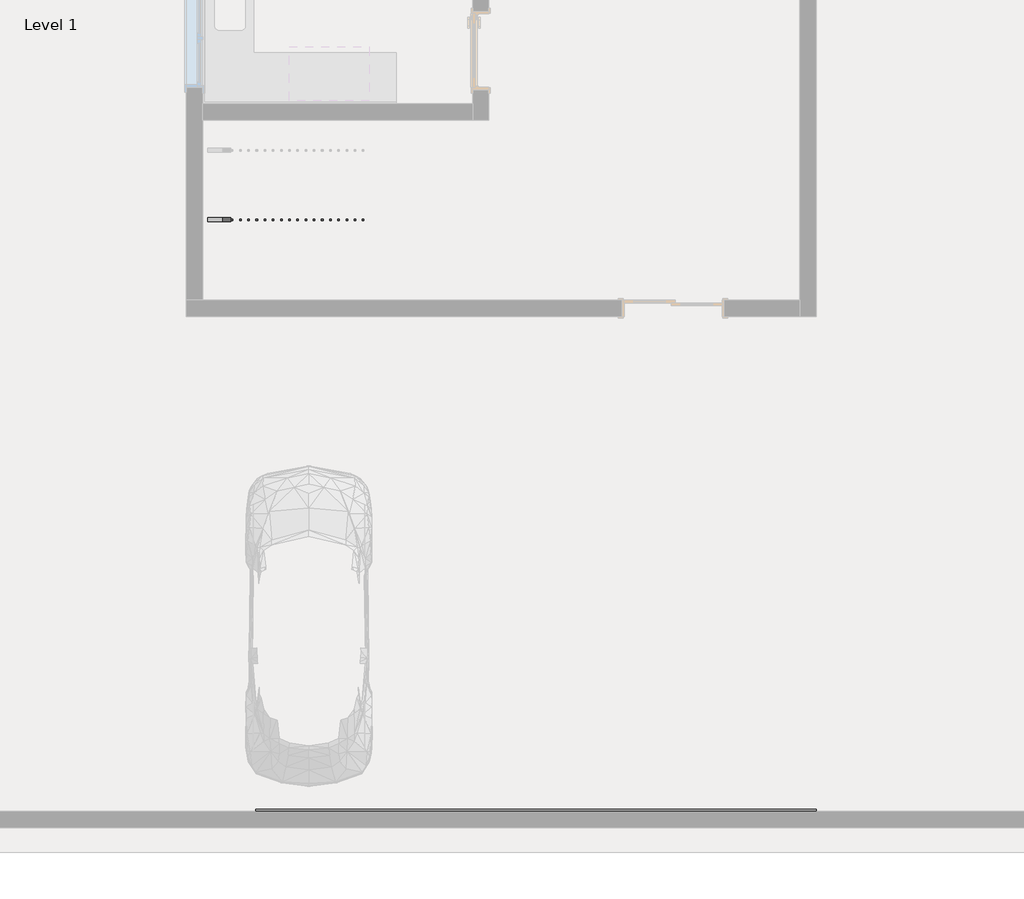
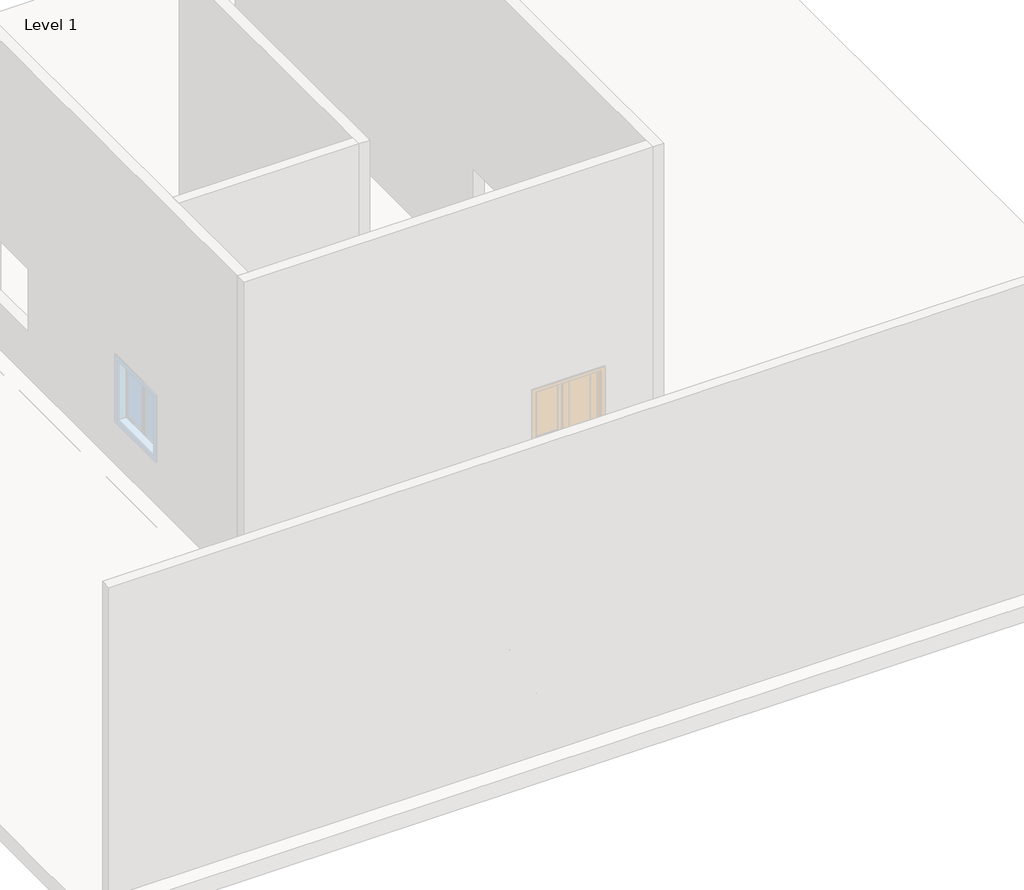
# One storey, part 2 of 3: 2 railings.
"""IFC4 building model written with IfcOpenShell, lengths in millimetres."""

from ifc_helpers import new_model, si_unit, frame, origin, origin_with_axes, place, context, project, spatial, polyline, outline, extrude, faceted_brep, element, save

model = new_model("IFC4")

# Units and contexts
model_context = context("Model", 3, world=origin())
ifc_project = project(units=[si_unit("LENGTHUNIT", "METRE", prefix="MILLI")], contexts=[model_context])

# Site, building, storey
site = spatial("IfcSite", under=ifc_project)
building = spatial("IfcBuilding", under=site)
storey = spatial("IfcBuildingStorey", under=building, Name="Level 1", Elevation=0.0)

# Railings
placement = place(None, origin())
element("IfcRailing", 1, ObjectType="Handrail - Rectangular", at=placement, inside=storey, context=model_context, shape_type="SolidModel", body=[
    faceted_brep([(-10833.7253666, -4140.9709044, 1090.3093851), (-10833.7253666, -4140.9709044, 1031.5187374), (-10833.7253666, -4191.7709044, 1031.5187374), (-10833.7253666, -4191.7709044, 1090.3093851), (-7938.1253666, -4140.9709044, 2777.0666667), (-7924.4080881, -4140.9709044, 2726.2666667), (-7924.4080881, -4191.7709044, 2726.2666667), (-7938.1253666, -4191.7709044, 2777.0666667), (-7499.9753666, -4140.9709044, 2777.0666667), (-7499.9753666, -4191.7709044, 2777.0666667), (-7449.1753666, -4191.7709044, 2726.2666667), (-7449.1753666, -4140.9709044, 2726.2666667)], [[[0, 1, 2, 3]], [[1, 0, 4, 5]], [[2, 1, 5, 6]], [[3, 2, 6, 7]], [[0, 3, 7, 4]], [[8, 9, 10, 11]], [[5, 4, 8, 11]], [[6, 5, 11, 10]], [[7, 6, 10, 9]], [[4, 7, 9, 8]]]),
    faceted_brep([(-7499.9753666, -4140.9709044, 2777.0666667), (-7499.9753666, -4090.1709044, 2777.0666667), (-7449.1753666, -4090.1709044, 2726.2666667), (-7449.1753666, -4140.9709044, 2726.2666667), (-7499.9753666, -4140.9709044, 3023.369697), (-7499.9753666, -4090.1709044, 2972.569697), (-7449.1753666, -4090.1709044, 2972.569697), (-7449.1753666, -4140.9709044, 3023.369697), (-7499.9753666, -4064.7709044, 3023.369697), (-7499.9753666, -4064.7709044, 2972.569697), (-7449.1753666, -4013.9709044, 2972.569697), (-7449.1753666, -4013.9709044, 3023.369697), (-7576.1753666, -4064.7709044, 3023.369697), (-7590.367776, -4064.7709044, 2972.569697), (-7590.367776, -4013.9709044, 2972.569697), (-7576.1753666, -4013.9709044, 3023.369697), (-9125.5753666, -4064.7709044, 3962.4), (-9125.5753666, -4013.9709044, 3962.4), (-9125.5753666, -4013.9709044, 3902.9985397), (-9125.5753666, -4064.7709044, 3902.9985397)], [[[0, 1, 2, 3]], [[1, 0, 4, 5]], [[2, 1, 5, 6]], [[3, 2, 6, 7]], [[0, 3, 7, 4]], [[5, 4, 8, 9]], [[6, 5, 9, 10]], [[7, 6, 10, 11]], [[4, 7, 11, 8]], [[9, 8, 12, 13]], [[10, 9, 13, 14]], [[11, 10, 14, 15]], [[8, 11, 15, 12]], [[16, 17, 18, 19]], [[13, 12, 16, 19]], [[14, 13, 19, 18]], [[15, 14, 18, 17]], [[12, 15, 17, 16]]]),
    extrude(outline(polyline([(3881.8318731, -9090.6503666), (3893.3773276, -9109.7003666), (2878.6666667, -9109.7003666), (2878.6666667, -9090.6503666), (3881.8318731, -9090.6503666)])), frame((0.0, -4048.8959044, 0.0), z_axis=(0.0, 1.0, 0.0), x_axis=(0.0, 0.0, 1.0)), (0.0, 0.0, 1.0), 19.05),
    extrude(outline(polyline([(3820.2561155, -8989.0503666), (3831.80157, -9008.1003666), (2878.6666667, -9008.1003666), (2878.6666667, -8989.0503666), (3820.2561155, -8989.0503666)])), frame((0.0, -4048.8959044, 0.0), z_axis=(0.0, 1.0, 0.0), x_axis=(0.0, 0.0, 1.0)), (0.0, 0.0, 1.0), 19.05),
    extrude(outline(polyline([(3758.6803579, -8887.4503666), (3770.2258125, -8906.5003666), (2878.6666667, -8906.5003666), (2878.6666667, -8887.4503666), (3758.6803579, -8887.4503666)])), frame((0.0, -4048.8959044, 0.0), z_axis=(0.0, 1.0, 0.0), x_axis=(0.0, 0.0, 1.0)), (0.0, 0.0, 1.0), 19.05),
    extrude(outline(polyline([(3697.1046004, -8785.8503666), (3708.6500549, -8804.9003666), (2709.3333333, -8804.9003666), (2709.3333333, -8785.8503666), (3697.1046004, -8785.8503666)])), frame((0.0, -4048.8959044, 0.0), z_axis=(0.0, 1.0, 0.0), x_axis=(0.0, 0.0, 1.0)), (0.0, 0.0, 1.0), 19.05),
    extrude(outline(polyline([(3635.5288428, -8684.2503666), (3647.0742973, -8703.3003666), (2709.3333333, -8703.3003666), (2709.3333333, -8684.2503666), (3635.5288428, -8684.2503666)])), frame((0.0, -4048.8959044, 0.0), z_axis=(0.0, 1.0, 0.0), x_axis=(0.0, 0.0, 1.0)), (0.0, 0.0, 1.0), 19.05),
    extrude(outline(polyline([(3573.9530852, -8582.6503666), (3585.4985397, -8601.7003666), (2709.3333333, -8601.7003666), (2709.3333333, -8582.6503666), (3573.9530852, -8582.6503666)])), frame((0.0, -4048.8959044, 0.0), z_axis=(0.0, 1.0, 0.0), x_axis=(0.0, 0.0, 1.0)), (0.0, 0.0, 1.0), 19.05),
    extrude(outline(polyline([(3512.3773276, -8481.0503666), (3523.9227822, -8500.1003666), (2540.0, -8500.1003666), (2540.0, -8481.0503666), (3512.3773276, -8481.0503666)])), frame((0.0, -4048.8959044, 0.0), z_axis=(0.0, 1.0, 0.0), x_axis=(0.0, 0.0, 1.0)), (0.0, 0.0, 1.0), 19.05),
    extrude(outline(polyline([(3450.80157, -8379.4503666), (3462.3470246, -8398.5003666), (2540.0, -8398.5003666), (2540.0, -8379.4503666), (3450.80157, -8379.4503666)])), frame((0.0, -4048.8959044, 0.0), z_axis=(0.0, 1.0, 0.0), x_axis=(0.0, 0.0, 1.0)), (0.0, 0.0, 1.0), 19.05),
    extrude(outline(polyline([(3389.2258125, -8277.8503666), (3400.771267, -8296.9003666), (2540.0, -8296.9003666), (2540.0, -8277.8503666), (3389.2258125, -8277.8503666)])), frame((0.0, -4048.8959044, 0.0), z_axis=(0.0, 1.0, 0.0), x_axis=(0.0, 0.0, 1.0)), (0.0, 0.0, 1.0), 19.05),
    extrude(outline(polyline([(3327.6500549, -8176.2503666), (3339.1955094, -8195.3003666), (2370.6666667, -8195.3003666), (2370.6666667, -8176.2503666), (3327.6500549, -8176.2503666)])), frame((0.0, -4048.8959044, 0.0), z_axis=(0.0, 1.0, 0.0), x_axis=(0.0, 0.0, 1.0)), (0.0, 0.0, 1.0), 19.05),
    extrude(outline(polyline([(3266.0742973, -8074.6503666), (3277.6197519, -8093.7003666), (2370.6666667, -8093.7003666), (2370.6666667, -8074.6503666), (3266.0742973, -8074.6503666)])), frame((0.0, -4048.8959044, 0.0), z_axis=(0.0, 1.0, 0.0), x_axis=(0.0, 0.0, 1.0)), (0.0, 0.0, 1.0), 19.05),
    extrude(outline(polyline([(3204.4985397, -7973.0503666), (3216.0439943, -7992.1003666), (2201.3333333, -7992.1003666), (2201.3333333, -7973.0503666), (3204.4985397, -7973.0503666)])), frame((0.0, -4048.8959044, 0.0), z_axis=(0.0, 1.0, 0.0), x_axis=(0.0, 0.0, 1.0)), (0.0, 0.0, 1.0), 19.05),
    extrude(outline(polyline([(3142.9227822, -7871.4503666), (3154.4682367, -7890.5003666), (2201.3333333, -7890.5003666), (2201.3333333, -7871.4503666), (3142.9227822, -7871.4503666)])), frame((0.0, -4048.8959044, 0.0), z_axis=(0.0, 1.0, 0.0), x_axis=(0.0, 0.0, 1.0)), (0.0, 0.0, 1.0), 19.05),
    extrude(outline(polyline([(3081.3470246, -7769.8503666), (3092.8924791, -7788.9003666), (2201.3333333, -7788.9003666), (2201.3333333, -7769.8503666), (3081.3470246, -7769.8503666)])), frame((0.0, -4048.8959044, 0.0), z_axis=(0.0, 1.0, 0.0), x_axis=(0.0, 0.0, 1.0)), (0.0, 0.0, 1.0), 19.05),
    extrude(outline(polyline([(3019.771267, -7668.2503666), (3031.3167216, -7687.3003666), (2032.0, -7687.3003666), (2032.0, -7668.2503666), (3019.771267, -7668.2503666)])), frame((0.0, -4048.8959044, 0.0), z_axis=(0.0, 1.0, 0.0), x_axis=(0.0, 0.0, 1.0)), (0.0, 0.0, 1.0), 19.05),
    extrude(outline(polyline([(-7566.6503666, -4029.8459044), (-7566.6503666, -4048.8959044), (-7585.7003666, -4048.8959044), (-7585.7003666, -4029.8459044), (-7566.6503666, -4029.8459044)])), frame((0.0, 0.0, 2032.0), z_axis=(0.0, 0.0, 1.0), x_axis=(1.0, 0.0, 0.0)), (0.0, 0.0, 1.0), 940.569697),
    extrude(outline(polyline([(-7465.0503666, -4074.2959044), (-7484.1003666, -4074.2959044), (-7484.1003666, -4055.2459044), (-7465.0503666, -4055.2459044), (-7465.0503666, -4074.2959044)])), frame((0.0, 0.0, 1862.6666667), z_axis=(0.0, 0.0, 1.0), x_axis=(1.0, 0.0, 0.0)), (0.0, 0.0, 1.0), 1109.9030303),
    extrude(outline(polyline([(-7541.2503666, -4175.8959044), (-7541.2503666, -4156.8459044), (-7522.2003666, -4156.8459044), (-7522.2003666, -4175.8959044), (-7541.2503666, -4175.8959044)])), frame((0.0, 0.0, 1862.6666667), z_axis=(0.0, 0.0, 1.0), x_axis=(1.0, 0.0, 0.0)), (0.0, 0.0, 1.0), 863.6),
    extrude(outline(polyline([(-7642.8503666, -4175.8959044), (-7642.8503666, -4156.8459044), (-7623.8003666, -4156.8459044), (-7623.8003666, -4175.8959044), (-7642.8503666, -4175.8959044)])), frame((0.0, 0.0, 1862.6666667), z_axis=(0.0, 0.0, 1.0), x_axis=(1.0, 0.0, 0.0)), (0.0, 0.0, 1.0), 863.6),
    extrude(outline(polyline([(-7744.4503666, -4175.8959044), (-7744.4503666, -4156.8459044), (-7725.4003666, -4156.8459044), (-7725.4003666, -4175.8959044), (-7744.4503666, -4175.8959044)])), frame((0.0, 0.0, 1862.6666667), z_axis=(0.0, 0.0, 1.0), x_axis=(1.0, 0.0, 0.0)), (0.0, 0.0, 1.0), 863.6),
    extrude(outline(polyline([(-7846.0503666, -4175.8959044), (-7846.0503666, -4156.8459044), (-7827.0003666, -4156.8459044), (-7827.0003666, -4175.8959044), (-7846.0503666, -4175.8959044)])), frame((0.0, 0.0, 1862.6666667), z_axis=(0.0, 0.0, 1.0), x_axis=(1.0, 0.0, 0.0)), (0.0, 0.0, 1.0), 863.6),
    extrude(outline(polyline([(2694.2323297, -7979.4003666), (2683.1352423, -7998.4503666), (1693.3333333, -7998.4503666), (1693.3333333, -7979.4003666), (2694.2323297, -7979.4003666)])), frame((0.0, -4175.8959044, 0.0), z_axis=(0.0, 1.0, 0.0), x_axis=(0.0, 0.0, 1.0)), (0.0, 0.0, 1.0), 19.05),
    extrude(outline(polyline([(2635.0478636, -8081.0003666), (2623.9507763, -8100.0503666), (1693.3333333, -8100.0503666), (1693.3333333, -8081.0003666), (2635.0478636, -8081.0003666)])), frame((0.0, -4175.8959044, 0.0), z_axis=(0.0, 1.0, 0.0), x_axis=(0.0, 0.0, 1.0)), (0.0, 0.0, 1.0), 19.05),
    extrude(outline(polyline([(2575.8633976, -8182.6003666), (2564.7663102, -8201.6503666), (1693.3333333, -8201.6503666), (1693.3333333, -8182.6003666), (2575.8633976, -8182.6003666)])), frame((0.0, -4175.8959044, 0.0), z_axis=(0.0, 1.0, 0.0), x_axis=(0.0, 0.0, 1.0)), (0.0, 0.0, 1.0), 19.05),
    extrude(outline(polyline([(2516.6789316, -8284.2003666), (2505.5818442, -8303.2503666), (1655.5210356, -8303.2503666), (1655.5210356, -8284.2003666), (2516.6789316, -8284.2003666)])), frame((0.0, -4175.8959044, 0.0), z_axis=(0.0, 1.0, 0.0), x_axis=(0.0, 0.0, 1.0)), (0.0, 0.0, 1.0), 19.05),
    extrude(outline(polyline([(2457.4944656, -8385.8003666), (2446.3973782, -8404.8503666), (1524.0, -8404.8503666), (1524.0, -8385.8003666), (2457.4944656, -8385.8003666)])), frame((0.0, -4175.8959044, 0.0), z_axis=(0.0, 1.0, 0.0), x_axis=(0.0, 0.0, 1.0)), (0.0, 0.0, 1.0), 19.05),
    extrude(outline(polyline([(2398.3099996, -8487.4003666), (2387.2129122, -8506.4503666), (1524.0, -8506.4503666), (1524.0, -8487.4003666), (2398.3099996, -8487.4003666)])), frame((0.0, -4175.8959044, 0.0), z_axis=(0.0, 1.0, 0.0), x_axis=(0.0, 0.0, 1.0)), (0.0, 0.0, 1.0), 19.05),
    extrude(outline(polyline([(2339.1255336, -8589.0003666), (2328.0284462, -8608.0503666), (1354.6666667, -8608.0503666), (1354.6666667, -8589.0003666), (2339.1255336, -8589.0003666)])), frame((0.0, -4175.8959044, 0.0), z_axis=(0.0, 1.0, 0.0), x_axis=(0.0, 0.0, 1.0)), (0.0, 0.0, 1.0), 19.05),
    extrude(outline(polyline([(2279.9410675, -8690.6003666), (2268.8439802, -8709.6503666), (1354.6666667, -8709.6503666), (1354.6666667, -8690.6003666), (2279.9410675, -8690.6003666)])), frame((0.0, -4175.8959044, 0.0), z_axis=(0.0, 1.0, 0.0), x_axis=(0.0, 0.0, 1.0)), (0.0, 0.0, 1.0), 19.05),
    extrude(outline(polyline([(2220.7566015, -8792.2003666), (2209.6595141, -8811.2503666), (1354.6666667, -8811.2503666), (1354.6666667, -8792.2003666), (2220.7566015, -8792.2003666)])), frame((0.0, -4175.8959044, 0.0), z_axis=(0.0, 1.0, 0.0), x_axis=(0.0, 0.0, 1.0)), (0.0, 0.0, 1.0), 19.05),
    extrude(outline(polyline([(2161.5721355, -8893.8003666), (2150.4750481, -8912.8503666), (1185.3333333, -8912.8503666), (1185.3333333, -8893.8003666), (2161.5721355, -8893.8003666)])), frame((0.0, -4175.8959044, 0.0), z_axis=(0.0, 1.0, 0.0), x_axis=(0.0, 0.0, 1.0)), (0.0, 0.0, 1.0), 19.05),
    extrude(outline(polyline([(2102.3876695, -8995.4003666), (2091.2905821, -9014.4503666), (1185.3333333, -9014.4503666), (1185.3333333, -8995.4003666), (2102.3876695, -8995.4003666)])), frame((0.0, -4175.8959044, 0.0), z_axis=(0.0, 1.0, 0.0), x_axis=(0.0, 0.0, 1.0)), (0.0, 0.0, 1.0), 19.05),
    extrude(outline(polyline([(2043.2032035, -9097.0003666), (2032.1061161, -9116.0503666), (1182.0453074, -9116.0503666), (1182.0453074, -9097.0003666), (2043.2032035, -9097.0003666)])), frame((0.0, -4175.8959044, 0.0), z_axis=(0.0, 1.0, 0.0), x_axis=(0.0, 0.0, 1.0)), (0.0, 0.0, 1.0), 19.05),
    extrude(outline(polyline([(1984.0187374, -9198.6003666), (1972.9216501, -9217.6503666), (1016.0, -9217.6503666), (1016.0, -9198.6003666), (1984.0187374, -9198.6003666)])), frame((0.0, -4175.8959044, 0.0), z_axis=(0.0, 1.0, 0.0), x_axis=(0.0, 0.0, 1.0)), (0.0, 0.0, 1.0), 19.05),
    extrude(outline(polyline([(1924.8342714, -9300.2003666), (1913.737184, -9319.2503666), (1016.0, -9319.2503666), (1016.0, -9300.2003666), (1924.8342714, -9300.2003666)])), frame((0.0, -4175.8959044, 0.0), z_axis=(0.0, 1.0, 0.0), x_axis=(0.0, 0.0, 1.0)), (0.0, 0.0, 1.0), 19.05),
    extrude(outline(polyline([(1865.6498054, -9401.8003666), (1854.552718, -9420.8503666), (1004.4919094, -9420.8503666), (1004.4919094, -9401.8003666), (1865.6498054, -9401.8003666)])), frame((0.0, -4175.8959044, 0.0), z_axis=(0.0, 1.0, 0.0), x_axis=(0.0, 0.0, 1.0)), (0.0, 0.0, 1.0), 19.05),
    extrude(outline(polyline([(1806.4653394, -9503.4003666), (1795.368252, -9522.4503666), (846.6666667, -9522.4503666), (846.6666667, -9503.4003666), (1806.4653394, -9503.4003666)])), frame((0.0, -4175.8959044, 0.0), z_axis=(0.0, 1.0, 0.0), x_axis=(0.0, 0.0, 1.0)), (0.0, 0.0, 1.0), 19.05),
    extrude(outline(polyline([(1747.2808734, -9605.0003666), (1736.183786, -9624.0503666), (846.6666667, -9624.0503666), (846.6666667, -9605.0003666), (1747.2808734, -9605.0003666)])), frame((0.0, -4175.8959044, 0.0), z_axis=(0.0, 1.0, 0.0), x_axis=(0.0, 0.0, 1.0)), (0.0, 0.0, 1.0), 19.05),
    extrude(outline(polyline([(1688.0964073, -9706.6003666), (1676.99932, -9725.6503666), (677.3333333, -9725.6503666), (677.3333333, -9706.6003666), (1688.0964073, -9706.6003666)])), frame((0.0, -4175.8959044, 0.0), z_axis=(0.0, 1.0, 0.0), x_axis=(0.0, 0.0, 1.0)), (0.0, 0.0, 1.0), 19.05),
    extrude(outline(polyline([(1628.9119413, -9808.2003666), (1617.8148539, -9827.2503666), (677.3333333, -9827.2503666), (677.3333333, -9808.2003666), (1628.9119413, -9808.2003666)])), frame((0.0, -4175.8959044, 0.0), z_axis=(0.0, 1.0, 0.0), x_axis=(0.0, 0.0, 1.0)), (0.0, 0.0, 1.0), 19.05),
    extrude(outline(polyline([(1569.7274753, -9909.8003666), (1558.6303879, -9928.8503666), (677.3333333, -9928.8503666), (677.3333333, -9909.8003666), (1569.7274753, -9909.8003666)])), frame((0.0, -4175.8959044, 0.0), z_axis=(0.0, 1.0, 0.0), x_axis=(0.0, 0.0, 1.0)), (0.0, 0.0, 1.0), 19.05),
    extrude(outline(polyline([(1510.5430093, -10011.4003666), (1499.4459219, -10030.4503666), (508.0, -10030.4503666), (508.0, -10011.4003666), (1510.5430093, -10011.4003666)])), frame((0.0, -4175.8959044, 0.0), z_axis=(0.0, 1.0, 0.0), x_axis=(0.0, 0.0, 1.0)), (0.0, 0.0, 1.0), 19.05),
    extrude(outline(polyline([(1451.3585433, -10113.0003666), (1440.2614559, -10132.0503666), (508.0, -10132.0503666), (508.0, -10113.0003666), (1451.3585433, -10113.0003666)])), frame((0.0, -4175.8959044, 0.0), z_axis=(0.0, 1.0, 0.0), x_axis=(0.0, 0.0, 1.0)), (0.0, 0.0, 1.0), 19.05),
    extrude(outline(polyline([(1392.1740772, -10214.6003666), (1381.0769899, -10233.6503666), (508.0, -10233.6503666), (508.0, -10214.6003666), (1392.1740772, -10214.6003666)])), frame((0.0, -4175.8959044, 0.0), z_axis=(0.0, 1.0, 0.0), x_axis=(0.0, 0.0, 1.0)), (0.0, 0.0, 1.0), 19.05),
    extrude(outline(polyline([(1332.9896112, -10316.2003666), (1321.8925238, -10335.2503666), (338.6666667, -10335.2503666), (338.6666667, -10316.2003666), (1332.9896112, -10316.2003666)])), frame((0.0, -4175.8959044, 0.0), z_axis=(0.0, 1.0, 0.0), x_axis=(0.0, 0.0, 1.0)), (0.0, 0.0, 1.0), 19.05),
    extrude(outline(polyline([(1273.8051452, -10417.8003666), (1262.7080578, -10436.8503666), (338.6666667, -10436.8503666), (338.6666667, -10417.8003666), (1273.8051452, -10417.8003666)])), frame((0.0, -4175.8959044, 0.0), z_axis=(0.0, 1.0, 0.0), x_axis=(0.0, 0.0, 1.0)), (0.0, 0.0, 1.0), 19.05),
    extrude(outline(polyline([(1214.6206792, -10519.4003666), (1203.5235918, -10538.4503666), (338.6666667, -10538.4503666), (338.6666667, -10519.4003666), (1214.6206792, -10519.4003666)])), frame((0.0, -4175.8959044, 0.0), z_axis=(0.0, 1.0, 0.0), x_axis=(0.0, 0.0, 1.0)), (0.0, 0.0, 1.0), 19.05),
    extrude(outline(polyline([(1155.4362132, -10621.0003666), (1144.3391258, -10640.0503666), (169.3333333, -10640.0503666), (169.3333333, -10621.0003666), (1155.4362132, -10621.0003666)])), frame((0.0, -4175.8959044, 0.0), z_axis=(0.0, 1.0, 0.0), x_axis=(0.0, 0.0, 1.0)), (0.0, 0.0, 1.0), 19.05),
    extrude(outline(polyline([(1096.2517471, -10722.6003666), (1085.1546598, -10741.6503666), (169.3333333, -10741.6503666), (169.3333333, -10722.6003666), (1096.2517471, -10722.6003666)])), frame((0.0, -4175.8959044, 0.0), z_axis=(0.0, 1.0, 0.0), x_axis=(0.0, 0.0, 1.0)), (0.0, 0.0, 1.0), 19.05),
    extrude(outline(polyline([(-7465.0503666, -4029.8459044), (-7465.0503666, -4048.8959044), (-7484.1003666, -4048.8959044), (-7484.1003666, -4029.8459044), (-7465.0503666, -4029.8459044)])), frame((0.0, 0.0, 1862.6666667), z_axis=(0.0, 0.0, 1.0), x_axis=(1.0, 0.0, 0.0)), (0.0, 0.0, 1.0), 1109.9030303),
    extrude(outline(polyline([(-7484.1003666, -4175.8959044), (-7484.1003666, -4156.8459044), (-7465.0503666, -4156.8459044), (-7465.0503666, -4175.8959044), (-7484.1003666, -4175.8959044)])), frame((0.0, 0.0, 1862.6666667), z_axis=(0.0, 0.0, 1.0), x_axis=(1.0, 0.0, 0.0)), (0.0, 0.0, 1.0), 863.6),
    extrude(outline(polyline([(-7947.6503666, -4175.8959044), (-7947.6503666, -4156.8459044), (-7928.6003666, -4156.8459044), (-7928.6003666, -4175.8959044), (-7947.6503666, -4175.8959044)])), frame((0.0, 0.0, 1862.6666667), z_axis=(0.0, 0.0, 1.0), x_axis=(1.0, 0.0, 0.0)), (0.0, 0.0, 1.0), 863.6),
    extrude(outline(polyline([(3891.4530852, -9106.5253666), (3902.9985397, -9125.5753666), (2878.6666667, -9125.5753666), (2878.6666667, -9106.5253666), (3891.4530852, -9106.5253666)])), frame((0.0, -4048.8959044, 0.0), z_axis=(0.0, 1.0, 0.0), x_axis=(0.0, 0.0, 1.0)), (0.0, 0.0, 1.0), 19.05),
    extrude(outline(polyline([(1042.6158248, -10814.6753666), (1031.5187374, -10833.7253666), (169.3333333, -10833.7253666), (169.3333333, -10814.6753666), (1042.6158248, -10814.6753666)])), frame((0.0, -4175.8959044, 0.0), z_axis=(0.0, 1.0, 0.0), x_axis=(0.0, 0.0, 1.0)), (0.0, 0.0, 1.0), 19.05),
])
element("IfcRailing", 2, ObjectType="Handrail - Rectangular", at=placement, inside=storey, context=model_context, shape_type="SweptSolid", body=[
    extrude(outline(polyline([(-10237.2260462, -11538.7818688), (-10237.2260462, -11487.9818688), (-3277.6260462, -11487.9818688), (-3277.6260462, -11538.7818688), (-10237.2260462, -11538.7818688)])), frame((0.0, 0.0, 863.6), z_axis=(0.0, 0.0, 1.0), x_axis=(1.0, 0.0, 0.0)), (0.0, 0.0, 1.0), 50.8),
    extrude(outline(polyline([(-3337.9510462, -11522.9068688), (-3337.9510462, -11503.8568688), (-3318.9010462, -11503.8568688), (-3318.9010462, -11522.9068688), (-3337.9510462, -11522.9068688)])), origin_with_axes(), (0.0, 0.0, 1.0), 863.6),
    extrude(outline(polyline([(-3439.5510462, -11522.9068688), (-3439.5510462, -11503.8568688), (-3420.5010462, -11503.8568688), (-3420.5010462, -11522.9068688), (-3439.5510462, -11522.9068688)])), origin_with_axes(), (0.0, 0.0, 1.0), 863.6),
    extrude(outline(polyline([(-3541.1510462, -11522.9068688), (-3541.1510462, -11503.8568688), (-3522.1010462, -11503.8568688), (-3522.1010462, -11522.9068688), (-3541.1510462, -11522.9068688)])), origin_with_axes(), (0.0, 0.0, 1.0), 863.6),
    extrude(outline(polyline([(-3642.7510462, -11522.9068688), (-3642.7510462, -11503.8568688), (-3623.7010462, -11503.8568688), (-3623.7010462, -11522.9068688), (-3642.7510462, -11522.9068688)])), origin_with_axes(), (0.0, 0.0, 1.0), 863.6),
    extrude(outline(polyline([(-3744.3510462, -11522.9068688), (-3744.3510462, -11503.8568688), (-3725.3010462, -11503.8568688), (-3725.3010462, -11522.9068688), (-3744.3510462, -11522.9068688)])), origin_with_axes(), (0.0, 0.0, 1.0), 863.6),
    extrude(outline(polyline([(-3845.9510462, -11522.9068688), (-3845.9510462, -11503.8568688), (-3826.9010462, -11503.8568688), (-3826.9010462, -11522.9068688), (-3845.9510462, -11522.9068688)])), origin_with_axes(), (0.0, 0.0, 1.0), 863.6),
    extrude(outline(polyline([(-3947.5510462, -11522.9068688), (-3947.5510462, -11503.8568688), (-3928.5010462, -11503.8568688), (-3928.5010462, -11522.9068688), (-3947.5510462, -11522.9068688)])), origin_with_axes(), (0.0, 0.0, 1.0), 863.6),
    extrude(outline(polyline([(-4049.1510462, -11522.9068688), (-4049.1510462, -11503.8568688), (-4030.1010462, -11503.8568688), (-4030.1010462, -11522.9068688), (-4049.1510462, -11522.9068688)])), origin_with_axes(), (0.0, 0.0, 1.0), 863.6),
    extrude(outline(polyline([(-4150.7510462, -11522.9068688), (-4150.7510462, -11503.8568688), (-4131.7010462, -11503.8568688), (-4131.7010462, -11522.9068688), (-4150.7510462, -11522.9068688)])), origin_with_axes(), (0.0, 0.0, 1.0), 863.6),
    extrude(outline(polyline([(-4252.3510462, -11522.9068688), (-4252.3510462, -11503.8568688), (-4233.3010462, -11503.8568688), (-4233.3010462, -11522.9068688), (-4252.3510462, -11522.9068688)])), origin_with_axes(), (0.0, 0.0, 1.0), 863.6),
    extrude(outline(polyline([(-4353.9510462, -11522.9068688), (-4353.9510462, -11503.8568688), (-4334.9010462, -11503.8568688), (-4334.9010462, -11522.9068688), (-4353.9510462, -11522.9068688)])), origin_with_axes(), (0.0, 0.0, 1.0), 863.6),
    extrude(outline(polyline([(-4455.5510462, -11522.9068688), (-4455.5510462, -11503.8568688), (-4436.5010462, -11503.8568688), (-4436.5010462, -11522.9068688), (-4455.5510462, -11522.9068688)])), origin_with_axes(), (0.0, 0.0, 1.0), 863.6),
    extrude(outline(polyline([(-4557.1510462, -11522.9068688), (-4557.1510462, -11503.8568688), (-4538.1010462, -11503.8568688), (-4538.1010462, -11522.9068688), (-4557.1510462, -11522.9068688)])), origin_with_axes(), (0.0, 0.0, 1.0), 863.6),
    extrude(outline(polyline([(-4658.7510462, -11522.9068688), (-4658.7510462, -11503.8568688), (-4639.7010462, -11503.8568688), (-4639.7010462, -11522.9068688), (-4658.7510462, -11522.9068688)])), origin_with_axes(), (0.0, 0.0, 1.0), 863.6),
    extrude(outline(polyline([(-4760.3510462, -11522.9068688), (-4760.3510462, -11503.8568688), (-4741.3010462, -11503.8568688), (-4741.3010462, -11522.9068688), (-4760.3510462, -11522.9068688)])), origin_with_axes(), (0.0, 0.0, 1.0), 863.6),
    extrude(outline(polyline([(-4861.9510462, -11522.9068688), (-4861.9510462, -11503.8568688), (-4842.9010462, -11503.8568688), (-4842.9010462, -11522.9068688), (-4861.9510462, -11522.9068688)])), origin_with_axes(), (0.0, 0.0, 1.0), 863.6),
    extrude(outline(polyline([(-4963.5510462, -11522.9068688), (-4963.5510462, -11503.8568688), (-4944.5010462, -11503.8568688), (-4944.5010462, -11522.9068688), (-4963.5510462, -11522.9068688)])), origin_with_axes(), (0.0, 0.0, 1.0), 863.6),
    extrude(outline(polyline([(-5065.1510462, -11522.9068688), (-5065.1510462, -11503.8568688), (-5046.1010462, -11503.8568688), (-5046.1010462, -11522.9068688), (-5065.1510462, -11522.9068688)])), origin_with_axes(), (0.0, 0.0, 1.0), 863.6),
    extrude(outline(polyline([(-5166.7510462, -11522.9068688), (-5166.7510462, -11503.8568688), (-5147.7010462, -11503.8568688), (-5147.7010462, -11522.9068688), (-5166.7510462, -11522.9068688)])), origin_with_axes(), (0.0, 0.0, 1.0), 863.6),
    extrude(outline(polyline([(-5268.3510462, -11522.9068688), (-5268.3510462, -11503.8568688), (-5249.3010462, -11503.8568688), (-5249.3010462, -11522.9068688), (-5268.3510462, -11522.9068688)])), origin_with_axes(), (0.0, 0.0, 1.0), 863.6),
    extrude(outline(polyline([(-5369.9510462, -11522.9068688), (-5369.9510462, -11503.8568688), (-5350.9010462, -11503.8568688), (-5350.9010462, -11522.9068688), (-5369.9510462, -11522.9068688)])), origin_with_axes(), (0.0, 0.0, 1.0), 863.6),
    extrude(outline(polyline([(-5471.5510462, -11522.9068688), (-5471.5510462, -11503.8568688), (-5452.5010462, -11503.8568688), (-5452.5010462, -11522.9068688), (-5471.5510462, -11522.9068688)])), origin_with_axes(), (0.0, 0.0, 1.0), 863.6),
    extrude(outline(polyline([(-5573.1510462, -11522.9068688), (-5573.1510462, -11503.8568688), (-5554.1010462, -11503.8568688), (-5554.1010462, -11522.9068688), (-5573.1510462, -11522.9068688)])), origin_with_axes(), (0.0, 0.0, 1.0), 863.6),
    extrude(outline(polyline([(-5674.7510462, -11522.9068688), (-5674.7510462, -11503.8568688), (-5655.7010462, -11503.8568688), (-5655.7010462, -11522.9068688), (-5674.7510462, -11522.9068688)])), origin_with_axes(), (0.0, 0.0, 1.0), 863.6),
    extrude(outline(polyline([(-5776.3510462, -11522.9068688), (-5776.3510462, -11503.8568688), (-5757.3010462, -11503.8568688), (-5757.3010462, -11522.9068688), (-5776.3510462, -11522.9068688)])), origin_with_axes(), (0.0, 0.0, 1.0), 863.6),
    extrude(outline(polyline([(-5877.9510462, -11522.9068688), (-5877.9510462, -11503.8568688), (-5858.9010462, -11503.8568688), (-5858.9010462, -11522.9068688), (-5877.9510462, -11522.9068688)])), origin_with_axes(), (0.0, 0.0, 1.0), 863.6),
    extrude(outline(polyline([(-5979.5510462, -11522.9068688), (-5979.5510462, -11503.8568688), (-5960.5010462, -11503.8568688), (-5960.5010462, -11522.9068688), (-5979.5510462, -11522.9068688)])), origin_with_axes(), (0.0, 0.0, 1.0), 863.6),
    extrude(outline(polyline([(-6081.1510462, -11522.9068688), (-6081.1510462, -11503.8568688), (-6062.1010462, -11503.8568688), (-6062.1010462, -11522.9068688), (-6081.1510462, -11522.9068688)])), origin_with_axes(), (0.0, 0.0, 1.0), 863.6),
    extrude(outline(polyline([(-6182.7510462, -11522.9068688), (-6182.7510462, -11503.8568688), (-6163.7010462, -11503.8568688), (-6163.7010462, -11522.9068688), (-6182.7510462, -11522.9068688)])), origin_with_axes(), (0.0, 0.0, 1.0), 863.6),
    extrude(outline(polyline([(-6284.3510462, -11522.9068688), (-6284.3510462, -11503.8568688), (-6265.3010462, -11503.8568688), (-6265.3010462, -11522.9068688), (-6284.3510462, -11522.9068688)])), origin_with_axes(), (0.0, 0.0, 1.0), 863.6),
    extrude(outline(polyline([(-6385.9510462, -11522.9068688), (-6385.9510462, -11503.8568688), (-6366.9010462, -11503.8568688), (-6366.9010462, -11522.9068688), (-6385.9510462, -11522.9068688)])), origin_with_axes(), (0.0, 0.0, 1.0), 863.6),
    extrude(outline(polyline([(-6487.5510462, -11522.9068688), (-6487.5510462, -11503.8568688), (-6468.5010462, -11503.8568688), (-6468.5010462, -11522.9068688), (-6487.5510462, -11522.9068688)])), origin_with_axes(), (0.0, 0.0, 1.0), 863.6),
    extrude(outline(polyline([(-6589.1510462, -11522.9068688), (-6589.1510462, -11503.8568688), (-6570.1010462, -11503.8568688), (-6570.1010462, -11522.9068688), (-6589.1510462, -11522.9068688)])), origin_with_axes(), (0.0, 0.0, 1.0), 863.6),
    extrude(outline(polyline([(-6690.7510462, -11522.9068688), (-6690.7510462, -11503.8568688), (-6671.7010462, -11503.8568688), (-6671.7010462, -11522.9068688), (-6690.7510462, -11522.9068688)])), origin_with_axes(), (0.0, 0.0, 1.0), 863.6),
    extrude(outline(polyline([(-6792.3510462, -11522.9068688), (-6792.3510462, -11503.8568688), (-6773.3010462, -11503.8568688), (-6773.3010462, -11522.9068688), (-6792.3510462, -11522.9068688)])), origin_with_axes(), (0.0, 0.0, 1.0), 863.6),
    extrude(outline(polyline([(-6893.9510462, -11522.9068688), (-6893.9510462, -11503.8568688), (-6874.9010462, -11503.8568688), (-6874.9010462, -11522.9068688), (-6893.9510462, -11522.9068688)])), origin_with_axes(), (0.0, 0.0, 1.0), 863.6),
    extrude(outline(polyline([(-6995.5510462, -11522.9068688), (-6995.5510462, -11503.8568688), (-6976.5010462, -11503.8568688), (-6976.5010462, -11522.9068688), (-6995.5510462, -11522.9068688)])), origin_with_axes(), (0.0, 0.0, 1.0), 863.6),
    extrude(outline(polyline([(-7097.1510462, -11522.9068688), (-7097.1510462, -11503.8568688), (-7078.1010462, -11503.8568688), (-7078.1010462, -11522.9068688), (-7097.1510462, -11522.9068688)])), origin_with_axes(), (0.0, 0.0, 1.0), 863.6),
    extrude(outline(polyline([(-7198.7510462, -11522.9068688), (-7198.7510462, -11503.8568688), (-7179.7010462, -11503.8568688), (-7179.7010462, -11522.9068688), (-7198.7510462, -11522.9068688)])), origin_with_axes(), (0.0, 0.0, 1.0), 863.6),
    extrude(outline(polyline([(-7300.3510462, -11522.9068688), (-7300.3510462, -11503.8568688), (-7281.3010462, -11503.8568688), (-7281.3010462, -11522.9068688), (-7300.3510462, -11522.9068688)])), origin_with_axes(), (0.0, 0.0, 1.0), 863.6),
    extrude(outline(polyline([(-7401.9510462, -11522.9068688), (-7401.9510462, -11503.8568688), (-7382.9010462, -11503.8568688), (-7382.9010462, -11522.9068688), (-7401.9510462, -11522.9068688)])), origin_with_axes(), (0.0, 0.0, 1.0), 863.6),
    extrude(outline(polyline([(-7503.5510462, -11522.9068688), (-7503.5510462, -11503.8568688), (-7484.5010462, -11503.8568688), (-7484.5010462, -11522.9068688), (-7503.5510462, -11522.9068688)])), origin_with_axes(), (0.0, 0.0, 1.0), 863.6),
    extrude(outline(polyline([(-7605.1510462, -11522.9068688), (-7605.1510462, -11503.8568688), (-7586.1010462, -11503.8568688), (-7586.1010462, -11522.9068688), (-7605.1510462, -11522.9068688)])), origin_with_axes(), (0.0, 0.0, 1.0), 863.6),
    extrude(outline(polyline([(-7706.7510462, -11522.9068688), (-7706.7510462, -11503.8568688), (-7687.7010462, -11503.8568688), (-7687.7010462, -11522.9068688), (-7706.7510462, -11522.9068688)])), origin_with_axes(), (0.0, 0.0, 1.0), 863.6),
    extrude(outline(polyline([(-7808.3510462, -11522.9068688), (-7808.3510462, -11503.8568688), (-7789.3010462, -11503.8568688), (-7789.3010462, -11522.9068688), (-7808.3510462, -11522.9068688)])), origin_with_axes(), (0.0, 0.0, 1.0), 863.6),
    extrude(outline(polyline([(-7909.9510462, -11522.9068688), (-7909.9510462, -11503.8568688), (-7890.9010462, -11503.8568688), (-7890.9010462, -11522.9068688), (-7909.9510462, -11522.9068688)])), origin_with_axes(), (0.0, 0.0, 1.0), 863.6),
    extrude(outline(polyline([(-8011.5510462, -11522.9068688), (-8011.5510462, -11503.8568688), (-7992.5010462, -11503.8568688), (-7992.5010462, -11522.9068688), (-8011.5510462, -11522.9068688)])), origin_with_axes(), (0.0, 0.0, 1.0), 863.6),
    extrude(outline(polyline([(-8113.1510462, -11522.9068688), (-8113.1510462, -11503.8568688), (-8094.1010462, -11503.8568688), (-8094.1010462, -11522.9068688), (-8113.1510462, -11522.9068688)])), origin_with_axes(), (0.0, 0.0, 1.0), 863.6),
    extrude(outline(polyline([(-8214.7510462, -11522.9068688), (-8214.7510462, -11503.8568688), (-8195.7010462, -11503.8568688), (-8195.7010462, -11522.9068688), (-8214.7510462, -11522.9068688)])), origin_with_axes(), (0.0, 0.0, 1.0), 863.6),
    extrude(outline(polyline([(-8316.3510462, -11522.9068688), (-8316.3510462, -11503.8568688), (-8297.3010462, -11503.8568688), (-8297.3010462, -11522.9068688), (-8316.3510462, -11522.9068688)])), origin_with_axes(), (0.0, 0.0, 1.0), 863.6),
    extrude(outline(polyline([(-8417.9510462, -11522.9068688), (-8417.9510462, -11503.8568688), (-8398.9010462, -11503.8568688), (-8398.9010462, -11522.9068688), (-8417.9510462, -11522.9068688)])), origin_with_axes(), (0.0, 0.0, 1.0), 863.6),
    extrude(outline(polyline([(-8519.5510462, -11522.9068688), (-8519.5510462, -11503.8568688), (-8500.5010462, -11503.8568688), (-8500.5010462, -11522.9068688), (-8519.5510462, -11522.9068688)])), origin_with_axes(), (0.0, 0.0, 1.0), 863.6),
    extrude(outline(polyline([(-8621.1510462, -11522.9068688), (-8621.1510462, -11503.8568688), (-8602.1010462, -11503.8568688), (-8602.1010462, -11522.9068688), (-8621.1510462, -11522.9068688)])), origin_with_axes(), (0.0, 0.0, 1.0), 863.6),
    extrude(outline(polyline([(-8722.7510462, -11522.9068688), (-8722.7510462, -11503.8568688), (-8703.7010462, -11503.8568688), (-8703.7010462, -11522.9068688), (-8722.7510462, -11522.9068688)])), origin_with_axes(), (0.0, 0.0, 1.0), 863.6),
    extrude(outline(polyline([(-8824.3510462, -11522.9068688), (-8824.3510462, -11503.8568688), (-8805.3010462, -11503.8568688), (-8805.3010462, -11522.9068688), (-8824.3510462, -11522.9068688)])), origin_with_axes(), (0.0, 0.0, 1.0), 863.6),
    extrude(outline(polyline([(-8925.9510462, -11522.9068688), (-8925.9510462, -11503.8568688), (-8906.9010462, -11503.8568688), (-8906.9010462, -11522.9068688), (-8925.9510462, -11522.9068688)])), origin_with_axes(), (0.0, 0.0, 1.0), 863.6),
    extrude(outline(polyline([(-9027.5510462, -11522.9068688), (-9027.5510462, -11503.8568688), (-9008.5010462, -11503.8568688), (-9008.5010462, -11522.9068688), (-9027.5510462, -11522.9068688)])), origin_with_axes(), (0.0, 0.0, 1.0), 863.6),
    extrude(outline(polyline([(-9129.1510462, -11522.9068688), (-9129.1510462, -11503.8568688), (-9110.1010462, -11503.8568688), (-9110.1010462, -11522.9068688), (-9129.1510462, -11522.9068688)])), origin_with_axes(), (0.0, 0.0, 1.0), 863.6),
    extrude(outline(polyline([(-9230.7510462, -11522.9068688), (-9230.7510462, -11503.8568688), (-9211.7010462, -11503.8568688), (-9211.7010462, -11522.9068688), (-9230.7510462, -11522.9068688)])), origin_with_axes(), (0.0, 0.0, 1.0), 863.6),
    extrude(outline(polyline([(-9332.3510462, -11522.9068688), (-9332.3510462, -11503.8568688), (-9313.3010462, -11503.8568688), (-9313.3010462, -11522.9068688), (-9332.3510462, -11522.9068688)])), origin_with_axes(), (0.0, 0.0, 1.0), 863.6),
    extrude(outline(polyline([(-9433.9510462, -11522.9068688), (-9433.9510462, -11503.8568688), (-9414.9010462, -11503.8568688), (-9414.9010462, -11522.9068688), (-9433.9510462, -11522.9068688)])), origin_with_axes(), (0.0, 0.0, 1.0), 863.6),
    extrude(outline(polyline([(-9535.5510462, -11522.9068688), (-9535.5510462, -11503.8568688), (-9516.5010462, -11503.8568688), (-9516.5010462, -11522.9068688), (-9535.5510462, -11522.9068688)])), origin_with_axes(), (0.0, 0.0, 1.0), 863.6),
    extrude(outline(polyline([(-9637.1510462, -11522.9068688), (-9637.1510462, -11503.8568688), (-9618.1010462, -11503.8568688), (-9618.1010462, -11522.9068688), (-9637.1510462, -11522.9068688)])), origin_with_axes(), (0.0, 0.0, 1.0), 863.6),
    extrude(outline(polyline([(-9738.7510462, -11522.9068688), (-9738.7510462, -11503.8568688), (-9719.7010462, -11503.8568688), (-9719.7010462, -11522.9068688), (-9738.7510462, -11522.9068688)])), origin_with_axes(), (0.0, 0.0, 1.0), 863.6),
    extrude(outline(polyline([(-9840.3510462, -11522.9068688), (-9840.3510462, -11503.8568688), (-9821.3010462, -11503.8568688), (-9821.3010462, -11522.9068688), (-9840.3510462, -11522.9068688)])), origin_with_axes(), (0.0, 0.0, 1.0), 863.6),
    extrude(outline(polyline([(-9941.9510462, -11522.9068688), (-9941.9510462, -11503.8568688), (-9922.9010462, -11503.8568688), (-9922.9010462, -11522.9068688), (-9941.9510462, -11522.9068688)])), origin_with_axes(), (0.0, 0.0, 1.0), 863.6),
    extrude(outline(polyline([(-10043.5510462, -11522.9068688), (-10043.5510462, -11503.8568688), (-10024.5010462, -11503.8568688), (-10024.5010462, -11522.9068688), (-10043.5510462, -11522.9068688)])), origin_with_axes(), (0.0, 0.0, 1.0), 863.6),
    extrude(outline(polyline([(-10145.1510462, -11522.9068688), (-10145.1510462, -11503.8568688), (-10126.1010462, -11503.8568688), (-10126.1010462, -11522.9068688), (-10145.1510462, -11522.9068688)])), origin_with_axes(), (0.0, 0.0, 1.0), 863.6),
    extrude(outline(polyline([(-3296.6760462, -11522.9068688), (-3296.6760462, -11503.8568688), (-3277.6260462, -11503.8568688), (-3277.6260462, -11522.9068688), (-3296.6760462, -11522.9068688)])), origin_with_axes(), (0.0, 0.0, 1.0), 863.6),
    extrude(outline(polyline([(-10237.2260462, -11522.9068688), (-10237.2260462, -11503.8568688), (-10218.1760462, -11503.8568688), (-10218.1760462, -11522.9068688), (-10237.2260462, -11522.9068688)])), origin_with_axes(), (0.0, 0.0, 1.0), 863.6),
])

save(model, "model.ifc")

# Revit data of these elements
# Type "Handrail - Rectangular"
#   Assembly Code = "C2010400"
#   built-in parameter 1008612 = 0.0416667 (stored number, unit not read)
#   built-in parameter 1008611 = 0.0416667 (stored number, unit not read)
#   built-in parameter 1008609 = 0.333333 (stored number, unit not read)
#   built-in parameter 1008604 = 0.166667 (stored number, unit not read)
#   built-in parameter 1008603 = 0.166667 (stored number, unit not read)
#   Railing Height = 3' - 0"
#   built-in parameter 1008630 = 2
#   built-in parameter 1008610 = 2
#   built-in parameter 1008618 = Baluster - Square : 3/4"
# Elements 1, 2 (IfcRailing, "Handrail - Rectangular")
#   Phase Created = New Construction
